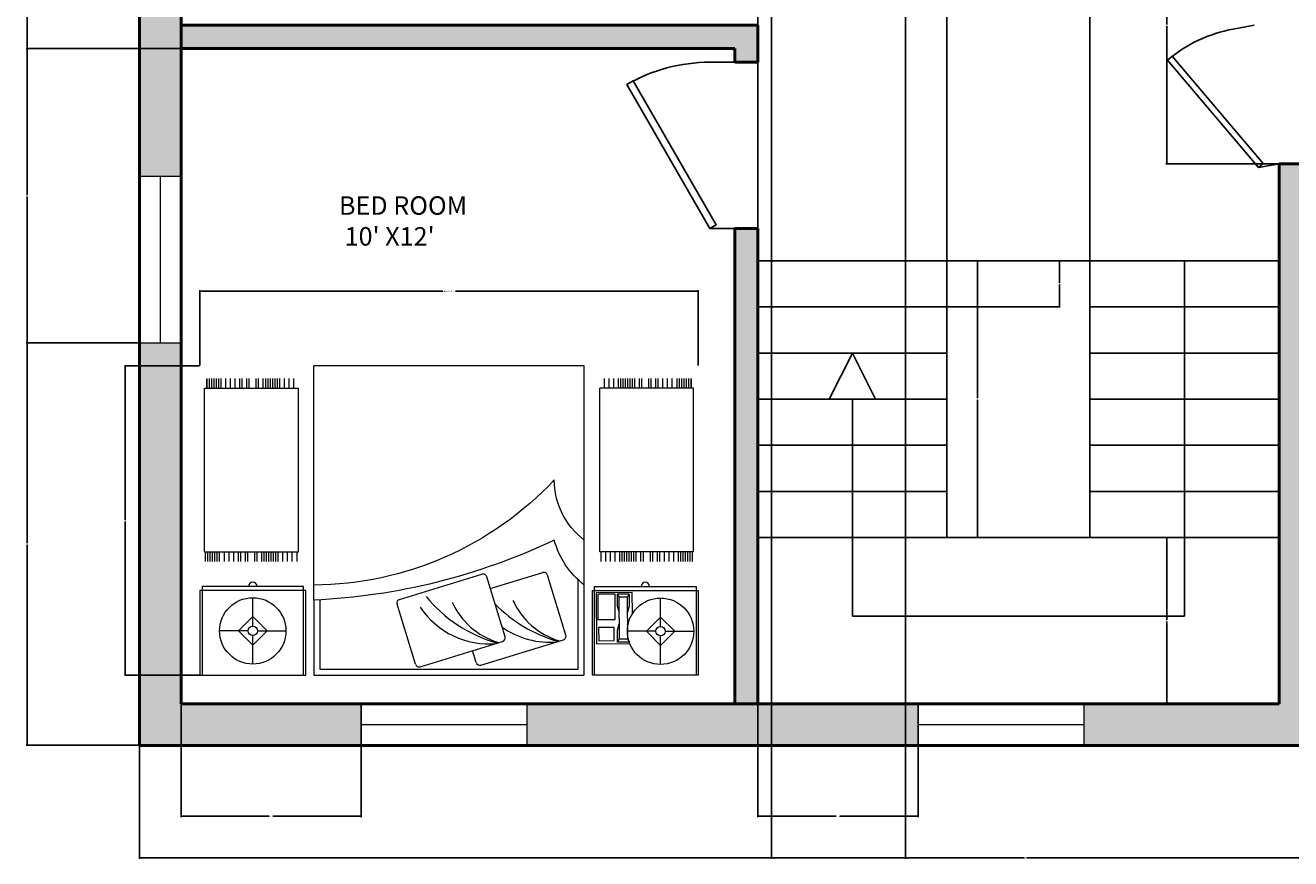
# Model space of a CAD drawing. Units: inches. Extents: x -23 to 411, y -22 to 507.
# Tile 1 of 5: x -23 to 252, y -22 to 159. Entities that reach past the tile are written whole.
import ezdxf

# ---------------------------------------------------------------- set-up
doc = ezdxf.new("R2010")
doc.units = ezdxf.units.IN
doc.header["$MEASUREMENT"] = 0
for name, color, linetype, lineweight in [('A-ANNO-DIMS', 2, 'Continuous', 18), ('A-AREA-IDEN', 7, 'Continuous', 25), ('A-FLOR-STRS', 7, 'Continuous', 25), ('A-WALL', 7, 'Continuous', 50), ('doors', 40, 'Continuous', 25), ('furniture', 220, 'Continuous', 18), ('window', 30, 'Continuous', 18)]:
    doc.layers.add(name, color=color, linetype=linetype, lineweight=lineweight)
doc.layers.add('A-WALL-PATT', color=179, linetype='Continuous', lineweight=13, true_color=0x161b4b)
doc.styles.get("Standard").update_dxf_attribs({"font": 'arial.ttf'})
doc.dimstyles.get("Standard").update_dxf_attribs({"dimtxt": 0.18, "dimasz": 0.18, "dimexe": 0.18, "dimexo": 0.0625, "dimgap": 0.09, "dimtad": 0, "dimtih": 1, "dimtoh": 1, "dimdec": 4, "dimzin": 0, "dimdsep": 46, "dimtxsty": 'Standard', "dimcen": 0.09, "dimadec": 0, "dimazin": 0, "dimtfac": 1, "dimtdec": 4, "dimtofl": 0, "dimtmove": 0, "dimatfit": 3, "dimfxl": 1, "dimtolj": 1, "dimtzin": 0, "dimarcsym": 0})

# ---------------------------------------------------------------- blocks, each defined once
blk = doc.blocks.new('*U6')
for p, q in [((0, 0), (0, -6)), ((40, 0), (40, -6))]:
    blk.add_line(p, q)
blk.add_lwpolyline([(0, 0), (34.64, 20), (35.52, 18.48), (0.87, -1.52)], close=True)
blk.add_arc((0, 0), 40, 0, 30)
blk = doc.blocks.new('3')
for p, q in [((185.8665, 224.6766), (185.8665, 225.2363)), ((185.8665, 225.2363), (186.566, 225.2363)), ((185.8805, 224.6487), (185.8805, 225.2363)), ((186.552, 225.2363), (186.552, 224.6487)), ((186.566, 225.2363), (186.566, 224.6766)), ((186.6199, 225.2363), (186.6199, 224.6399)), ((188.4089, 225.2363), (186.6199, 225.2363)), ((188.4089, 224.7393), (188.4089, 225.2363)), ((188.4627, 225.2363), (188.4627, 224.6766)), ((189.1623, 225.2363), (188.4627, 225.2363)), ((188.4767, 225.2363), (188.4767, 224.6486)), ((189.1483, 224.6486), (189.1483, 225.2363)), ((189.1623, 224.6766), (189.1623, 225.2363)), ((186.1157, 225.1643), (186.1157, 224.9763)), ((187.3034, 225.1683), (186.7581, 225.0015)), ((187.7059, 225.1793), (187.1607, 225.0124)), ((187.3344, 225.1518), (187.3586, 225.073)), ((187.737, 225.1628), (187.8585, 224.7657)), ((188.8125, 225.1618), (188.8125, 224.9738)), ((186.0216, 224.9449), (186.1157, 225.0389)), ((186.1157, 225.0389), (186.2097, 224.9449)), ((186.5397, 225.0274), (186.3193, 225.0266)), ((186.3215, 225.0167), (186.4008, 225.017)), ((186.3334, 224.9969), (186.3215, 225.0167)), ((186.3334, 224.9969), (186.389, 224.9971)), ((186.334, 224.858), (186.3334, 224.9969)), ((186.4008, 225.017), (186.389, 224.9971)), ((186.3895, 224.8582), (186.389, 224.9971)), ((186.4008, 225.017), (186.4011, 224.9376)), ((186.5409, 224.6901), (186.5397, 225.0274)), ((186.7416, 224.9704), (186.8631, 224.5734)), ((187.1442, 224.9814), (187.2657, 224.5843)), ((188.8125, 225.0365), (188.7185, 224.9424)), ((188.9065, 224.9424), (188.8125, 225.0365)), ((186.0843, 224.9449), (185.8963, 224.9449)), ((186.1157, 224.8509), (186.0216, 224.9449)), ((186.2097, 224.9449), (186.1157, 224.8509)), ((186.1157, 224.9136), (186.1157, 224.7256)), ((186.147, 224.9449), (186.335, 224.9449)), ((186.3314, 224.9055), (186.3338, 224.8977)), ((186.4011, 224.9376), (186.3894, 224.8979)), ((188.7812, 224.9424), (188.5931, 224.9424)), ((188.7185, 224.9424), (188.8125, 224.8484)), ((188.8125, 224.8484), (188.9065, 224.9424)), ((188.8125, 224.9111), (188.8125, 224.723)), ((188.8438, 224.9424), (189.0319, 224.9424)), ((186.3023, 224.8297), (186.3029, 224.6892)), ((186.3224, 224.7786), (186.3341, 224.8183)), ((186.334, 224.858), (186.3345, 224.7191)), ((186.3895, 224.8582), (186.39, 224.7193)), ((186.4017, 224.7789), (186.3897, 224.8185)), ((186.3227, 224.6992), (186.3224, 224.7786)), ((186.3345, 224.7191), (186.3227, 224.6992)), ((186.3345, 224.7191), (186.39, 224.7193)), ((186.402, 224.6995), (186.39, 224.7193)), ((186.402, 224.6995), (186.4017, 224.7789)), ((187.842, 224.7347), (187.2967, 224.5678)), ((188.4089, 224.7393), (188.4089, 223.1907)), ((186.566, 224.6766), (185.8665, 224.6766)), ((186.552, 224.6487), (185.8805, 224.6487)), ((186.3029, 224.6892), (186.5409, 224.6901)), ((186.3227, 224.6992), (186.402, 224.6995)), ((186.6199, 224.6399), (186.6199, 223.1907)), ((187.2416, 224.6632), (186.8942, 224.5569)), ((188.4627, 224.6766), (189.1623, 224.6766)), ((188.4767, 224.6486), (189.1483, 224.6486)), ((185.904, 224.4849, -0.9094), (185.904, 224.4204, -0.9094)), ((185.9195, 224.4849, -0.9094), (185.9195, 224.4204, -0.9094)), ((185.9195, 224.4849, -0.9094), (185.9195, 224.4204, -0.9094)), ((185.935, 224.4849, -0.9094), (185.935, 224.4204, -0.9094)), ((185.9505, 224.4849, -0.9094), (185.9505, 224.4204, -0.9094)), ((185.966, 224.4849, -0.9094), (185.966, 224.4204, -0.9094)), ((185.9815, 224.4849, -0.9094), (185.9815, 224.4204, -0.9094)), ((185.997, 224.4849, -0.9094), (185.997, 224.4204, -0.9094)), ((186.028, 224.4849, -0.9094), (186.028, 224.4204, -0.9094)), ((186.059, 224.4849, -0.9094), (186.059, 224.4204, -0.9094)), ((186.09, 224.4849, -0.9094), (186.09, 224.4204, -0.9094)), ((186.09, 224.4849, -0.9094), (186.09, 224.4204, -0.9094)), ((186.121, 224.4849, -0.9094), (186.121, 224.4204, -0.9094)), ((186.1365, 224.4849, -0.9094), (186.1365, 224.4204, -0.9094)), ((186.1675, 224.4849, -0.9094), (186.1675, 224.4204, -0.9094)), ((186.183, 224.4849, -0.9094), (186.183, 224.4204, -0.9094)), ((186.2295, 224.4849, -0.9094), (186.2295, 224.4204, -0.9094)), ((186.245, 224.4849, -0.9094), (186.245, 224.4204, -0.9094)), ((186.276, 224.4849, -0.9094), (186.276, 224.4204, -0.9094)), ((186.2915, 224.4849, -0.9094), (186.2915, 224.4204, -0.9094)), ((186.307, 224.4849, -0.9094), (186.307, 224.4204, -0.9094)), ((186.3225, 224.4849, -0.9094), (186.3225, 224.4204, -0.9094)), ((186.338, 224.4849, -0.9094), (186.338, 224.4204, -0.9094)), ((186.3535, 224.4849, -0.9094), (186.3535, 224.4204, -0.9094)), ((186.369, 224.4849, -0.9094), (186.369, 224.4204, -0.9094)), ((186.3845, 224.4849, -0.9094), (186.3845, 224.4204, -0.9094)), ((186.4155, 224.4849, -0.9094), (186.4155, 224.4204, -0.9094)), ((186.4465, 224.4849, -0.9094), (186.4465, 224.4204, -0.9094)), ((186.4775, 224.4849, -0.9094), (186.4775, 224.4204, -0.9094)), ((186.5085, 224.4849, -0.9094), (186.5085, 224.4204, -0.9094)), ((188.5202, 224.4849, -0.9094), (188.5202, 224.4204, -0.9094)), ((188.5512, 224.4849, -0.9094), (188.5512, 224.4204, -0.9094)), ((188.5822, 224.4849, -0.9094), (188.5822, 224.4204, -0.9094)), ((188.6132, 224.4849, -0.9094), (188.6132, 224.4204, -0.9094)), ((188.6442, 224.4849, -0.9094), (188.6442, 224.4204, -0.9094)), ((188.6597, 224.4849, -0.9094), (188.6597, 224.4204, -0.9094)), ((188.6752, 224.4849, -0.9094), (188.6752, 224.4204, -0.9094)), ((188.6907, 224.4849, -0.9094), (188.6907, 224.4204, -0.9094)), ((188.7062, 224.4849, -0.9094), (188.7062, 224.4204, -0.9094)), ((188.7217, 224.4849, -0.9094), (188.7217, 224.4204, -0.9094)), ((188.7372, 224.4849, -0.9094), (188.7372, 224.4204, -0.9094)), ((188.7527, 224.4849, -0.9094), (188.7527, 224.4204, -0.9094)), ((188.7837, 224.4849, -0.9094), (188.7837, 224.4204, -0.9094)), ((188.7992, 224.4849, -0.9094), (188.7992, 224.4204, -0.9094)), ((188.8457, 224.4849, -0.9094), (188.8457, 224.4204, -0.9094)), ((188.8612, 224.4849, -0.9094), (188.8612, 224.4204, -0.9094)), ((188.8922, 224.4849, -0.9094), (188.8922, 224.4204, -0.9094)), ((188.9077, 224.4849, -0.9094), (188.9077, 224.4204, -0.9094)), ((188.9387, 224.4849, -0.9094), (188.9387, 224.4204, -0.9094)), ((188.9387, 224.4849, -0.9094), (188.9387, 224.4204, -0.9094)), ((188.9697, 224.4849, -0.9094), (188.9697, 224.4204, -0.9094)), ((189.0007, 224.4849, -0.9094), (189.0007, 224.4204, -0.9094)), ((189.0317, 224.4849, -0.9094), (189.0317, 224.4204, -0.9094)), ((189.0472, 224.4849, -0.9094), (189.0472, 224.4204, -0.9094)), ((189.0627, 224.4849, -0.9094), (189.0627, 224.4204, -0.9094)), ((189.0782, 224.4849, -0.9094), (189.0782, 224.4204, -0.9094)), ((189.0937, 224.4849, -0.9094), (189.0937, 224.4204, -0.9094)), ((189.1092, 224.4849, -0.9094), (189.1092, 224.4204, -0.9094)), ((189.1092, 224.4849, -0.9094), (189.1092, 224.4204, -0.9094)), ((189.1247, 224.4849, -0.9094), (189.1247, 224.4204, -0.9094)), ((185.8974, 224.4204, -0.9094), (185.8974, 223.3378, -0.9094)), ((185.8974, 224.4204, -0.9094), (186.5174, 224.4204, -0.9094)), ((186.5174, 224.4204, -0.9094), (186.5174, 223.3378, -0.9094)), ((189.1313, 224.4204, -0.9094), (188.5113, 224.4204, -0.9094)), ((188.5113, 224.4204, -0.9094), (188.5113, 223.3378, -0.9094)), ((189.1313, 224.4204, -0.9094), (189.1313, 223.3378, -0.9094)), ((185.8974, 223.3378, -0.9094), (186.5174, 223.3378, -0.9094)), ((185.9114, 223.3378, -0.9094), (185.9114, 223.2789, -0.9094)), ((185.9114, 223.3378, -0.9094), (185.9114, 223.2789, -0.9094)), ((185.9114, 223.3378, -0.9094), (185.9114, 223.2789, -0.9094)), ((185.9138, 223.3378, -0.9094), (185.9138, 223.2732, -0.9094)), ((185.9293, 223.3378, -0.9094), (185.9293, 223.2732, -0.9094)), ((185.9293, 223.3378, -0.9094), (185.9293, 223.2732, -0.9094)), ((185.9448, 223.3378, -0.9094), (185.9448, 223.2732, -0.9094)), ((185.9603, 223.3378, -0.9094), (185.9603, 223.2732, -0.9094)), ((185.9758, 223.3378, -0.9094), (185.9758, 223.2732, -0.9094)), ((185.9913, 223.3378, -0.9094), (185.9913, 223.2732, -0.9094)), ((186.0068, 223.3378, -0.9094), (186.0068, 223.2732, -0.9094)), ((186.0378, 223.3378, -0.9094), (186.0378, 223.2732, -0.9094)), ((186.0688, 223.3378, -0.9094), (186.0688, 223.2732, -0.9094)), ((186.0998, 223.3378, -0.9094), (186.0998, 223.2732, -0.9094)), ((186.0998, 223.3378, -0.9094), (186.0998, 223.2732, -0.9094)), ((186.1308, 223.3378, -0.9094), (186.1308, 223.2732, -0.9094)), ((186.1463, 223.3378, -0.9094), (186.1463, 223.2732, -0.9094)), ((186.1773, 223.3378, -0.9094), (186.1773, 223.2732, -0.9094)), ((186.1928, 223.3378, -0.9094), (186.1928, 223.2732, -0.9094)), ((186.2393, 223.3378, -0.9094), (186.2393, 223.2732, -0.9094)), ((186.2548, 223.3378, -0.9094), (186.2548, 223.2732, -0.9094)), ((186.2858, 223.3378, -0.9094), (186.2858, 223.2732, -0.9094)), ((186.3013, 223.3378, -0.9094), (186.3013, 223.2732, -0.9094)), ((186.3168, 223.3378, -0.9094), (186.3168, 223.2732, -0.9094)), ((186.3323, 223.3378, -0.9094), (186.3323, 223.2732, -0.9094)), ((186.3478, 223.3378, -0.9094), (186.3478, 223.2732, -0.9094)), ((186.3633, 223.3378, -0.9094), (186.3633, 223.2732, -0.9094)), ((186.3788, 223.3378, -0.9094), (186.3788, 223.2732, -0.9094)), ((186.3943, 223.3378, -0.9094), (186.3943, 223.2732, -0.9094)), ((186.4253, 223.3378, -0.9094), (186.4253, 223.2732, -0.9094)), ((186.4563, 223.3378, -0.9094), (186.4563, 223.2732, -0.9094)), ((186.4873, 223.3378, -0.9094), (186.4873, 223.2732, -0.9094)), ((189.1313, 223.3378, -0.9094), (188.5113, 223.3378, -0.9094)), ((188.5414, 223.3378, -0.9094), (188.5414, 223.2732, -0.9094)), ((188.5724, 223.3378, -0.9094), (188.5724, 223.2732, -0.9094)), ((188.6034, 223.3378, -0.9094), (188.6034, 223.2732, -0.9094)), ((188.6344, 223.3378, -0.9094), (188.6344, 223.2732, -0.9094)), ((188.6499, 223.3378, -0.9094), (188.6499, 223.2732, -0.9094)), ((188.6654, 223.3378, -0.9094), (188.6654, 223.2732, -0.9094)), ((188.6809, 223.3378, -0.9094), (188.6809, 223.2732, -0.9094)), ((188.6964, 223.3378, -0.9094), (188.6964, 223.2732, -0.9094)), ((188.7119, 223.3378, -0.9094), (188.7119, 223.2732, -0.9094)), ((188.7274, 223.3378, -0.9094), (188.7274, 223.2732, -0.9094)), ((188.7429, 223.3378, -0.9094), (188.7429, 223.2732, -0.9094)), ((188.7739, 223.3378, -0.9094), (188.7739, 223.2732, -0.9094)), ((188.7894, 223.3378, -0.9094), (188.7894, 223.2732, -0.9094)), ((188.8359, 223.3378, -0.9094), (188.8359, 223.2732, -0.9094)), ((188.8514, 223.3378, -0.9094), (188.8514, 223.2732, -0.9094)), ((188.8824, 223.3378, -0.9094), (188.8824, 223.2732, -0.9094)), ((188.8979, 223.3378, -0.9094), (188.8979, 223.2732, -0.9094)), ((188.9289, 223.3378, -0.9094), (188.9289, 223.2732, -0.9094)), ((188.9289, 223.3378, -0.9094), (188.9289, 223.2732, -0.9094)), ((188.9599, 223.3378, -0.9094), (188.9599, 223.2732, -0.9094)), ((188.9909, 223.3378, -0.9094), (188.9909, 223.2732, -0.9094)), ((189.022, 223.3378, -0.9094), (189.022, 223.2732, -0.9094)), ((189.0375, 223.3378, -0.9094), (189.0375, 223.2732, -0.9094)), ((189.053, 223.3378, -0.9094), (189.053, 223.2732, -0.9094)), ((189.0685, 223.3378, -0.9094), (189.0685, 223.2732, -0.9094)), ((189.084, 223.3378, -0.9094), (189.084, 223.2732, -0.9094)), ((189.0995, 223.3378, -0.9094), (189.0995, 223.2732, -0.9094)), ((189.0995, 223.3378, -0.9094), (189.0995, 223.2732, -0.9094)), ((189.115, 223.3378, -0.9094), (189.115, 223.2732, -0.9094)), ((189.1173, 223.3378, -0.9094), (189.1173, 223.2789, -0.9094)), ((189.1173, 223.3378, -0.9094), (189.1173, 223.2789, -0.9094)), ((189.1173, 223.3378, -0.9094), (189.1173, 223.2789, -0.9094)), ((186.6199, 223.1907), (188.4089, 223.1907))]:
    blk.add_line(p, q)
blk.add_lwpolyline([(188.3691, 224.7374), (188.3691, 225.1965), (186.6596, 225.1965), (186.6596, 224.606)])
for points in [[(186.4217, 225.0072), (186.422, 224.9199), (186.5252, 224.9202), (186.5249, 225.0075)], [(186.4153, 224.8663), (186.4159, 224.6996), (186.531, 224.7), (186.5304, 224.8667)]]:
    blk.add_lwpolyline(points, close=True)
for points in [[(186.6199, 224.6399, -0.162278), (186.8186, 224.3418, -0.100664), (188.4089, 224.7393, -0.100664)], [(186.6199, 224.3418, -0.236068), (186.8186, 223.9442, -0.205258), (188.4089, 224.6399, -0.205258)]]:
    blk.add_lwpolyline(points, format="xyb")
for centre, radius in [((186.1157, 224.9449), 0.2194), ((188.8125, 224.9424), 0.2194), ((186.1157, 224.9449), 0.0313), ((188.8125, 224.9424), 0.0313)]:
    blk.add_circle(centre, radius)
for centre, radius, start, end in [((187.3107, 225.1446), 0.0248, 17.0142, 107.0142), ((187.7132, 225.1555), 0.0248, 17.0142, 107.0142), ((186.7654, 224.9777), 0.0248, 107.0142, 197.0142), ((186.6474, 224.5408), 0.4873, 24.22087, 73.06906), ((186.8477, 224.4712), 0.5468, 54.68511, 95.16051), ((186.5359, 224.1054), 0.9426, 44.27274, 73.71889), ((187.1679, 224.9887), 0.0248, 107.0142, 197.0142), ((187.0499, 224.5517), 0.4873, 24.22087, 73.06906), ((187.2502, 224.4821), 0.5468, 33.78007, 95.16051), ((186.9385, 224.1164), 0.9426, 39.40233, 73.71889), ((187.8347, 224.7585), 0.0248, 287.0142, 17.0142), ((186.2163, 224.6487), 0.028, 180, 0), ((188.8125, 224.6486), 0.028, 180, 0), ((186.8869, 224.5806), 0.0248, 197.0142, 287.0142), ((187.2894, 224.5916), 0.0248, 197.0142, 287.0142)]:
    blk.add_arc(centre, radius, start, end)
blk = doc.blocks.new('WIN-36IN')
for p, q in [((9, 36), (0, 36)), ((0, 36), (0, 0)), ((4.5, 0), (4.5, 36)), ((9, 0), (9, 36)), ((0, 0), (9, 0)), ((0, 0), (4.5, 0))]:
    blk.add_line(p, q)
blk = doc.blocks.new('*D16')
at = {"layer": 'A-ANNO-DIMS', "color": 0, "lineweight": -2, "transparency": 16777216}
for p, q in [((15.27, 85.16), (15.27, 101.48)), ((123.27, 85.16), (123.27, 101.48)), ((15.45, 101.3), (67.88, 101.3)), ((123.09, 101.3), (70.65, 101.3))]:
    blk.add_line(p, q, dxfattribs=at)
at = {"layer": 'A-ANNO-DIMS', "color": 0, "transparency": 16777216}
for points in [[(15.45, 101.33), (15.45, 101.27), (15.27, 101.3)], [(123.09, 101.33), (123.09, 101.27), (123.27, 101.3)]]:
    blk.add_solid(points, dxfattribs=at)
at = {"layer": 'Defpoints', "color": 0, "transparency": 16777216}
for p in [(15.27, 101.3), (15.27, 85.1), (123.27, 85.1)]:
    blk.add_point(p, dxfattribs=at)
at = {"layer": 'A-ANNO-DIMS', "color": 0, "transparency": 16777216, "insert": (69.27, 101.3), "char_height": 0.18, "attachment_point": 5}
blk.add_mtext('\\A1;BED GROUP 108 TYP.', dxfattribs=at)
blk = doc.blocks.new('*D17')
at = {"layer": 'A-ANNO-DIMS', "color": 0, "lineweight": -2, "transparency": 16777216}
for p, q in [((15.2, 85.1), (-1.11, 85.1)), ((-0.93, 84.92), (-0.93, 51.77)), ((-0.93, 18.25), (-0.93, 51.4)), ((15.2, 18.07), (-1.11, 18.07))]:
    blk.add_line(p, q, dxfattribs=at)
at = {"layer": 'A-ANNO-DIMS', "color": 0, "transparency": 16777216}
for points in [[(-0.96, 84.92), (-0.9, 84.92), (-0.93, 85.1)], [(-0.96, 18.25), (-0.9, 18.25), (-0.93, 18.07)]]:
    blk.add_solid(points, dxfattribs=at)
at = {"layer": 'Defpoints', "color": 0, "transparency": 16777216}
for p in [(15.27, 85.1), (-0.93, 18.07), (15.27, 18.07)]:
    blk.add_point(p, dxfattribs=at)
at = {"layer": 'A-ANNO-DIMS', "color": 0, "transparency": 16777216, "insert": (-0.93, 51.59), "char_height": 0.18, "attachment_point": 5}
blk.add_mtext('\\A1;67 TYP.', dxfattribs=at)
blk = doc.blocks.new('*D28')
at = {"layer": 'A-ANNO-DIMS', "color": 0, "lineweight": -2, "transparency": 16777216}
for p, q in [((2.17, 2.83), (2.17, -21.66)), ((386.17, 2.83), (386.17, -21.66)), ((2.35, -21.48), (193.89, -21.48)), ((385.99, -21.48), (194.46, -21.48))]:
    blk.add_line(p, q, dxfattribs=at)
at = {"layer": 'A-ANNO-DIMS', "color": 0, "transparency": 16777216}
for points in [[(2.35, -21.45), (2.35, -21.51), (2.17, -21.48)], [(385.99, -21.45), (385.99, -21.51), (386.17, -21.48)]]:
    blk.add_solid(points, dxfattribs=at)
at = {"layer": 'Defpoints', "color": 0, "transparency": 16777216}
for p in [(2.17, 2.9), (386.17, 2.9), (386.17, -21.48)]:
    blk.add_point(p, dxfattribs=at)
at = {"layer": 'A-ANNO-DIMS', "color": 0, "transparency": 16777216, "insert": (194.17, -21.48), "char_height": 0.18, "attachment_point": 5}
blk.add_mtext('\\A1;384', dxfattribs=at)
blk = doc.blocks.new('*D38')
at = {"layer": 'A-ANNO-DIMS', "color": 0, "lineweight": -2, "transparency": 16777216}
for p, q in [((2.11, 90.12), (-22.38, 90.12)), ((-22.2, 89.94), (-22.2, 46.69)), ((-22.2, 3.08), (-22.2, 46.33)), ((2.11, 2.9), (-22.38, 2.9))]:
    blk.add_line(p, q, dxfattribs=at)
at = {"layer": 'A-ANNO-DIMS', "color": 0, "transparency": 16777216}
for points in [[(-22.23, 89.94), (-22.17, 89.94), (-22.2, 90.12)], [(-22.23, 3.08), (-22.17, 3.08), (-22.2, 2.9)]]:
    blk.add_solid(points, dxfattribs=at)
at = {"layer": 'Defpoints', "color": 0, "transparency": 16777216}
for p in [(-22.2, 90.12), (2.17, 90.12), (2.17, 2.9)]:
    blk.add_point(p, dxfattribs=at)
at = {"layer": 'A-ANNO-DIMS', "color": 0, "transparency": 16777216, "insert": (-22.2, 46.51), "char_height": 0.18, "attachment_point": 5}
blk.add_mtext('\\A1;87.22', dxfattribs=at)
blk = doc.blocks.new('*D39')
at = {"layer": 'A-ANNO-DIMS', "color": 0, "lineweight": -2, "transparency": 16777216}
for p, q in [((11.11, 153.9), (-22.38, 153.9)), ((-22.2, 153.72), (-22.2, 122.19)), ((-22.2, 90.3), (-22.2, 121.83)), ((2.11, 90.12), (-22.38, 90.12))]:
    blk.add_line(p, q, dxfattribs=at)
at = {"layer": 'A-ANNO-DIMS', "color": 0, "transparency": 16777216}
for points in [[(-22.23, 153.72), (-22.17, 153.72), (-22.2, 153.9)], [(-22.23, 90.3), (-22.17, 90.3), (-22.2, 90.12)]]:
    blk.add_solid(points, dxfattribs=at)
at = {"layer": 'Defpoints', "color": 0, "transparency": 16777216}
for p in [(-22.2, 153.9), (11.17, 153.9), (2.17, 90.12)]:
    blk.add_point(p, dxfattribs=at)
at = {"layer": 'A-ANNO-DIMS', "color": 0, "transparency": 16777216, "insert": (-22.2, 122.01), "char_height": 0.18, "attachment_point": 5}
blk.add_mtext('\\A1;63.78', dxfattribs=at)
blk = doc.blocks.new('*D40')
at = {"layer": 'A-ANNO-DIMS', "color": 0, "lineweight": -2, "transparency": 16777216}
for p, q in [((2.11, 176.25), (-22.38, 176.25)), ((-22.2, 176.07), (-22.2, 165.26)), ((-22.2, 154.08), (-22.2, 164.89)), ((11.11, 153.9), (-22.38, 153.9))]:
    blk.add_line(p, q, dxfattribs=at)
at = {"layer": 'A-ANNO-DIMS', "color": 0, "transparency": 16777216}
for points in [[(-22.23, 176.07), (-22.17, 176.07), (-22.2, 176.25)], [(-22.23, 154.08), (-22.17, 154.08), (-22.2, 153.9)]]:
    blk.add_solid(points, dxfattribs=at)
at = {"layer": 'Defpoints', "color": 0, "transparency": 16777216}
for p in [(-22.2, 176.25), (2.17, 176.25), (11.17, 153.9)]:
    blk.add_point(p, dxfattribs=at)
at = {"layer": 'A-ANNO-DIMS', "color": 0, "transparency": 16777216, "insert": (-22.2, 165.08), "char_height": 0.18, "attachment_point": 5}
blk.add_mtext('\\A1;22.358', dxfattribs=at)
blk = doc.blocks.new('*D45')
at = {"layer": 'A-ANNO-DIMS', "color": 0, "lineweight": -2, "transparency": 16777216}
for p, q in [((136.17, 107.96), (136.17, 507.45)), ((177.17, 107.96), (177.17, 507.45)), ((136.35, 507.27), (156.47, 507.27)), ((176.99, 507.27), (156.88, 507.27))]:
    blk.add_line(p, q, dxfattribs=at)
at = {"layer": 'A-ANNO-DIMS', "color": 0, "transparency": 16777216}
for points in [[(136.35, 507.3), (136.35, 507.24), (136.17, 507.27)], [(176.99, 507.3), (176.99, 507.24), (177.17, 507.27)]]:
    blk.add_solid(points, dxfattribs=at)
at = {"layer": 'Defpoints', "color": 0, "transparency": 16777216}
for p in [(177.17, 507.27), (136.17, 107.9), (177.17, 107.9)]:
    blk.add_point(p, dxfattribs=at)
at = {"layer": 'A-ANNO-DIMS', "color": 0, "transparency": 16777216, "insert": (156.67, 507.27), "char_height": 0.18, "attachment_point": 5}
blk.add_mtext('\\A1;41', dxfattribs=at)
blk = doc.blocks.new('*D46')
at = {"layer": 'A-ANNO-DIMS', "color": 0, "lineweight": -2, "transparency": 16777216}
for p, q in [((177.17, 107.96), (177.17, 507.45)), ((208.17, 107.96), (208.17, 507.45)), ((177.35, 507.27), (192.47, 507.27)), ((207.99, 507.27), (192.88, 507.27))]:
    blk.add_line(p, q, dxfattribs=at)
at = {"layer": 'A-ANNO-DIMS', "color": 0, "transparency": 16777216}
for points in [[(177.35, 507.3), (177.35, 507.24), (177.17, 507.27)], [(207.99, 507.3), (207.99, 507.24), (208.17, 507.27)]]:
    blk.add_solid(points, dxfattribs=at)
at = {"layer": 'Defpoints', "color": 0, "transparency": 16777216}
for p in [(208.17, 507.27), (177.17, 107.9), (208.17, 107.9)]:
    blk.add_point(p, dxfattribs=at)
at = {"layer": 'A-ANNO-DIMS', "color": 0, "transparency": 16777216, "insert": (192.67, 507.27), "char_height": 0.18, "attachment_point": 5}
blk.add_mtext('\\A1;31', dxfattribs=at)
blk = doc.blocks.new('*D47')
at = {"layer": 'A-ANNO-DIMS', "color": 0, "lineweight": -2, "transparency": 16777216}
for p, q in [((208.11, 107.9), (183.62, 107.9)), ((183.8, 107.72), (183.8, 78.08)), ((183.8, 48.08), (183.8, 77.72)), ((208.11, 47.9), (183.62, 47.9))]:
    blk.add_line(p, q, dxfattribs=at)
at = {"layer": 'A-ANNO-DIMS', "color": 0, "transparency": 16777216}
for points in [[(183.77, 107.72), (183.83, 107.72), (183.8, 107.9)], [(183.77, 48.08), (183.83, 48.08), (183.8, 47.9)]]:
    blk.add_solid(points, dxfattribs=at)
at = {"layer": 'Defpoints', "color": 0, "transparency": 16777216}
for p in [(183.8, 107.9), (208.17, 107.9), (208.17, 47.9)]:
    blk.add_point(p, dxfattribs=at)
at = {"layer": 'A-ANNO-DIMS', "color": 0, "transparency": 16777216, "insert": (183.8, 77.9), "char_height": 0.18, "attachment_point": 5}
blk.add_mtext('\\A1;60', dxfattribs=at)
blk = doc.blocks.new('*D48')
at = {"layer": 'A-ANNO-DIMS', "color": 0, "lineweight": -2, "transparency": 16777216}
for p, q in [((177.24, 107.9), (201.73, 107.9)), ((201.55, 107.72), (201.55, 103.08)), ((201.55, 98.08), (201.55, 102.72)), ((177.24, 97.9), (201.73, 97.9))]:
    blk.add_line(p, q, dxfattribs=at)
at = {"layer": 'A-ANNO-DIMS', "color": 0, "transparency": 16777216}
for points in [[(201.52, 107.72), (201.58, 107.72), (201.55, 107.9)], [(201.52, 98.08), (201.58, 98.08), (201.55, 97.9)]]:
    blk.add_solid(points, dxfattribs=at)
at = {"layer": 'Defpoints', "color": 0, "transparency": 16777216}
for p in [(177.17, 107.9), (177.17, 97.9), (201.55, 97.9)]:
    blk.add_point(p, dxfattribs=at)
at = {"layer": 'A-ANNO-DIMS', "color": 0, "transparency": 16777216, "insert": (201.55, 102.9), "char_height": 0.18, "attachment_point": 5}
blk.add_mtext('\\A1;10', dxfattribs=at)
blk = doc.blocks.new('*D49')
at = {"layer": 'A-ANNO-DIMS', "color": 0, "lineweight": -2, "transparency": 16777216}
for p, q in [((249.11, 47.9), (224.62, 47.9)), ((224.8, 47.72), (224.8, 30.08)), ((224.8, 12.08), (224.8, 29.72)), ((249.11, 11.9), (224.62, 11.9))]:
    blk.add_line(p, q, dxfattribs=at)
at = {"layer": 'A-ANNO-DIMS', "color": 0, "transparency": 16777216}
for points in [[(224.77, 47.72), (224.83, 47.72), (224.8, 47.9)], [(224.77, 12.08), (224.83, 12.08), (224.8, 11.9)]]:
    blk.add_solid(points, dxfattribs=at)
at = {"layer": 'Defpoints', "color": 0, "transparency": 16777216}
for p in [(224.8, 47.9), (249.17, 47.9), (249.17, 11.9)]:
    blk.add_point(p, dxfattribs=at)
at = {"layer": 'A-ANNO-DIMS', "color": 0, "transparency": 16777216, "insert": (224.8, 29.9), "char_height": 0.18, "attachment_point": 5}
blk.add_mtext('\\A1;36', dxfattribs=at)
blk = doc.blocks.new('*D50')
at = {"layer": 'A-ANNO-DIMS', "color": 0, "lineweight": -2, "transparency": 16777216}
for p, q in [((139.17, 372.83), (139.17, -21.66)), ((168.17, 372.83), (168.17, -21.66)), ((139.35, -21.48), (153.45, -21.48)), ((167.99, -21.48), (153.9, -21.48))]:
    blk.add_line(p, q, dxfattribs=at)
at = {"layer": 'A-ANNO-DIMS', "color": 0, "transparency": 16777216}
for points in [[(139.35, -21.45), (139.35, -21.51), (139.17, -21.48)], [(167.99, -21.45), (167.99, -21.51), (168.17, -21.48)]]:
    blk.add_solid(points, dxfattribs=at)
at = {"layer": 'Defpoints', "color": 0, "transparency": 16777216}
for p in [(139.17, 372.9), (168.17, 372.9), (168.17, -21.48)]:
    blk.add_point(p, dxfattribs=at)
at = {"layer": 'A-ANNO-DIMS', "color": 0, "transparency": 16777216, "insert": (153.67, -21.48), "char_height": 0.18, "attachment_point": 5}
blk.add_mtext('\\A1;29', dxfattribs=at)
blk = doc.blocks.new('*D52')
at = {"layer": 'A-ANNO-DIMS', "color": 0, "lineweight": -2, "transparency": 16777216}
for p, q in [((249.11, 188.9), (224.62, 188.9)), ((224.8, 188.72), (224.8, 159.08)), ((224.8, 129.08), (224.8, 158.72)), ((249.11, 128.9), (224.62, 128.9))]:
    blk.add_line(p, q, dxfattribs=at)
at = {"layer": 'A-ANNO-DIMS', "color": 0, "transparency": 16777216}
for points in [[(224.77, 188.72), (224.83, 188.72), (224.8, 188.9)], [(224.77, 129.08), (224.83, 129.08), (224.8, 128.9)]]:
    blk.add_solid(points, dxfattribs=at)
at = {"layer": 'Defpoints', "color": 0, "transparency": 16777216}
for p in [(224.8, 188.9), (249.17, 188.9), (249.17, 128.9)]:
    blk.add_point(p, dxfattribs=at)
at = {"layer": 'A-ANNO-DIMS', "color": 0, "transparency": 16777216, "insert": (224.8, 158.9), "char_height": 0.18, "attachment_point": 5}
blk.add_mtext('\\A1;60', dxfattribs=at)
blk = doc.blocks.new('*D58')
at = {"layer": 'A-ANNO-DIMS', "color": 0, "lineweight": -2, "transparency": 16777216}
for p, q in [((11.17, 11.83), (11.17, -12.66)), ((50.21, 11.83), (50.21, -12.66)), ((11.35, -12.48), (30.3, -12.48)), ((50.03, -12.48), (31.09, -12.48))]:
    blk.add_line(p, q, dxfattribs=at)
at = {"layer": 'A-ANNO-DIMS', "color": 0, "transparency": 16777216}
for points in [[(11.35, -12.45), (11.35, -12.51), (11.17, -12.48)], [(50.03, -12.45), (50.03, -12.51), (50.21, -12.48)]]:
    blk.add_solid(points, dxfattribs=at)
at = {"layer": 'Defpoints', "color": 0, "transparency": 16777216}
for p in [(11.17, 11.9), (50.21, 11.9), (11.17, -12.48)]:
    blk.add_point(p, dxfattribs=at)
at = {"layer": 'A-ANNO-DIMS', "color": 0, "transparency": 16777216, "insert": (30.69, -12.48), "char_height": 0.18, "attachment_point": 5}
blk.add_mtext('\\A1;39.04', dxfattribs=at)
blk = doc.blocks.new('*D59')
at = {"layer": 'A-ANNO-DIMS', "color": 0, "lineweight": -2, "transparency": 16777216}
for p, q in [((136.17, 11.83), (136.17, -12.66)), ((170.92, 11.83), (170.92, -12.66)), ((136.35, -12.48), (153.15, -12.48)), ((170.74, -12.48), (153.94, -12.48))]:
    blk.add_line(p, q, dxfattribs=at)
at = {"layer": 'A-ANNO-DIMS', "color": 0, "transparency": 16777216}
for points in [[(136.35, -12.45), (136.35, -12.51), (136.17, -12.48)], [(170.74, -12.45), (170.74, -12.51), (170.92, -12.48)]]:
    blk.add_solid(points, dxfattribs=at)
at = {"layer": 'Defpoints', "color": 0, "transparency": 16777216}
for p in [(136.17, 11.9), (170.92, 11.9), (136.17, -12.48)]:
    blk.add_point(p, dxfattribs=at)
at = {"layer": 'A-ANNO-DIMS', "color": 0, "transparency": 16777216, "insert": (153.55, -12.48), "char_height": 0.18, "attachment_point": 5}
blk.add_mtext('\\A1;34.74', dxfattribs=at)

msp = doc.modelspace()

# ---------------------------------------------------------------- hatches: boundary and pattern name
at = {"layer": 'A-WALL-PATT'}
h = msp.add_hatch(color=256, dxfattribs=at)
h.dxf.hatch_style = 1
h.paths.add_polyline_path([(37.3453, 482.8972), (2.1746, 482.8972), (2.1746, 414.9823), (11.1746, 414.9823), (11.1746, 473.8972), (37.3453, 473.8972)])
h.paths.add_polyline_path([(149.2817, 482.8972), (73.3453, 482.8972), (73.3453, 473.8972), (131.1746, 473.8972), (131.1746, 356.8972), (136.1746, 356.8972), (136.1746, 372.8972), (139.1746, 372.8972), (139.1746, 377.8972), (136.1746, 377.8972), (136.1746, 473.8972), (149.2817, 473.8972)])
h.paths.add_polyline_path([(209.1361, 482.8972), (173.2817, 482.8972), (173.2817, 473.8972), (190.1746, 473.8972), (190.1746, 377.8972), (168.1746, 377.8972), (168.1746, 372.8972), (249.1746, 372.8972), (249.1746, 356.8972), (254.1746, 356.8972), (254.1746, 380.8972), (249.1746, 380.8972), (249.1746, 377.8972), (195.1746, 377.8972), (195.1746, 473.8972), (209.1361, 473.8972)])
h.paths.add_polyline_path([(309.9724, 482.8972), (233.1361, 482.8972), (233.1361, 473.8972), (249.1746, 473.8972), (249.1746, 409.8972), (254.1746, 409.8972), (254.1746, 473.8972), (309.9724, 473.8972)])
h.paths.add_polyline_path([(386.1746, 482.8972), (345.9724, 482.8972), (345.9724, 473.8972), (377.1746, 473.8972), (377.1746, 445.6454), (386.1746, 445.6454)])
h.paths.add_polyline_path([(386.1746, 409.6454), (377.1746, 409.6454), (377.1746, 317.8972), (254.1746, 317.8972), (254.1746, 320.8972), (249.1746, 320.8972), (249.1746, 317.8972), (249.1746, 235.8972), (254.1746, 235.8972), (254.1746, 312.8972), (377.1746, 312.8972), (377.1746, 281.3732), (386.1746, 281.3732)])
h.paths.add_polyline_path([(386.1746, 245.3732), (377.1746, 245.3732), (377.1746, 196.8972), (254.1746, 196.8972), (254.1746, 199.8972), (249.1746, 199.8972), (249.1746, 196.8972), (249.1746, 188.8972), (254.1746, 188.8972), (254.1746, 191.8972), (264.1746, 191.8972), (377.1746, 191.8972), (377.1746, 11.8972), (377.1746, 2.8972), (386.1746, 2.8972)])
h.paths.add_polyline_path([(254.1746, 128.8972), (249.1746, 128.8972), (249.1746, 11.8972), (206.9157, 11.8972), (206.9157, 2.8972), (254.1746, 2.8972)])
h.paths.add_polyline_path([(170.9157, 11.8972), (86.2116, 11.8972), (86.2116, 2.8972), (170.9157, 2.8972)])
h.paths.add_polyline_path([(136.1746, 114.8972), (131.1746, 114.8972), (131.1746, 11.8972), (136.1746, 11.8972)])
h.paths.add_polyline_path([(50.2116, 11.8972), (11.1746, 11.8972), (11.1746, 90.1201), (2.1746, 90.1201), (2.1746, 2.8972), (50.2116, 2.8972)])
h.paths.add_polyline_path([(11.1746, 176.2548), (2.1746, 176.2548), (2.1746, 126.1201), (11.1746, 126.1201)])
h.paths.add_polyline_path([(136.1746, 158.8972), (11.1746, 158.8972), (11.1746, 153.8972), (131.1746, 153.8972), (131.1746, 150.8972), (136.1746, 150.8972)])
h.paths.add_polyline_path([(11.1746, 269.5052), (2.1746, 269.5052), (2.1746, 212.2548), (11.1746, 212.2548)])
h.paths.add_polyline_path([(11.1746, 378.9823), (2.1746, 378.9823), (2.1746, 305.5052), (11.1746, 305.5052), (11.1746, 312.8972), (136.1746, 312.8972), (136.1746, 320.8972), (131.1746, 320.8972), (131.1746, 317.8972), (11.1746, 317.8972)])

# ---------------------------------------------------------------- linework, layer by layer
at = {"layer": 'A-FLOR-STRS'}
for p, q in [((136.1746, 107.8972), (177.1746, 107.8972)), ((136.1746, 107.8972), (177.1746, 107.8972)), ((177.1746, 107.8972), (177.1746, 47.8972)), ((208.1746, 107.8972), (249.1746, 107.8972)), ((249.1746, 107.8972), (208.1746, 107.8972)), ((208.1746, 107.8972), (208.1746, 47.8972)), ((228.6746, 107.8972), (228.6746, 35.3776)), ((136.1746, 97.8972), (177.1746, 97.8972)), ((208.1746, 97.8972), (249.1746, 97.8972)), ((136.1746, 87.8972), (177.1746, 87.8972)), ((151.6746, 77.8972), (156.6746, 87.8972)), ((161.6746, 77.8972), (156.6746, 87.8972)), ((208.1746, 87.8972), (249.1746, 87.8972)), ((136.1746, 77.8972), (177.1746, 77.8972)), ((136.1746, 77.8972), (177.1746, 77.8972)), ((156.6746, 77.8972), (151.6746, 77.8972)), ((156.6746, 77.8972), (156.6746, 47.8972)), ((156.6746, 77.8972), (161.6746, 77.8972)), ((208.1746, 77.8972), (249.1746, 77.8972)), ((208.1746, 77.8972), (249.1746, 77.8972)), ((136.1746, 67.8972), (177.1746, 67.8972)), ((208.1746, 67.8972), (249.1746, 67.8972)), ((136.1746, 57.8972), (177.1746, 57.8972)), ((208.1746, 57.8972), (249.1746, 57.8972)), ((136.1746, 11.8972), (136.1746, 47.8972)), ((136.1746, 47.8972), (249.1746, 47.8972)), ((156.6746, 47.8972), (156.6746, 30.8972)), ((228.6746, 30.8972), (228.6746, 35.3776)), ((156.6746, 30.8972), (228.6746, 30.8972))]:
    msp.add_line(p, q, dxfattribs=at)
at = {"layer": 'A-WALL'}
for p, q in [((11.1746, 11.8972), (11.1746, 191.8972)), ((11.1746, 158.8972), (136.1746, 158.8972)), ((136.1746, 150.8972), (136.1746, 158.8972)), ((11.1746, 153.8972), (131.1746, 153.8972)), ((131.1746, 150.8972), (131.1746, 153.8972)), ((131.1746, 153.8972), (131.1746, 150.8972)), ((131.1746, 150.8972), (136.1746, 150.8972)), ((249.1746, 11.8972), (249.1746, 128.8972)), ((249.1746, 128.8972), (254.1746, 128.8972)), ((131.1746, 11.8972), (131.1746, 114.8972)), ((136.1746, 114.8972), (131.1746, 114.8972)), ((136.1746, 11.8972), (136.1746, 114.8972)), ((249.1746, 11.8972), (11.1746, 11.8972))]:
    msp.add_line(p, q, dxfattribs=at)
msp.add_lwpolyline([(254.1746, 2.8972), (2.1746, 2.8972), (2.1746, 482.8972), (386.1746, 482.8972), (386.1746, 2.8972), (377.1746, 2.8972)], dxfattribs=at)

# ---------------------------------------------------------------- block references
at = {"layer": 'doors'}
for p, xscale, yscale, zscale, rotation in [((244.6746, 128.0817), 0.7622159057711964, 0.7622159057711964, 0.7622159057711964, 100.2717207928814), ((125.7746, 114.8972), 0.9, 0.9, 0.9, 90)]:
    msp.add_blockref('*U6', p, dxfattribs=dict(at, xscale=xscale, yscale=yscale, zscale=zscale, rotation=rotation))
at = {"layer": 'furniture', "xscale": 32.76894482774335, "yscale": 32.76894482774335, "zscale": 32.76894482774335, "rotation": 180}
msp.add_blockref('3', (6213.9154, 7398.8253), dxfattribs=at)
at = {"layer": 'window'}
for p, rotation in [((11.1741, 126.1203), 180), ((50.2114, 11.8967), 270), ((170.9155, 11.8967), 270)]:
    msp.add_blockref('WIN-36IN', p, dxfattribs=dict(at, rotation=rotation))

# ---------------------------------------------------------------- texts
at = {"layer": 'A-AREA-IDEN', "insert": (45.4014, 121.8448), "char_height": 4, "attachment_point": 1}
msp.add_mtext_dynamic_manual_height_columns("BED ROOM\\P 10' X12'", width=61.991846, gutter_width=1, heights=[0], dxfattribs=at)

# ---------------------------------------------------------------- dimensions: what is measured, and where the dimension line sits
at = {"layer": 'A-ANNO-DIMS'}
for base, p1, p2, picture, middle in [((177.1746, 507.2747), (136.1746, 107.8972), (177.1746, 107.8972), '*D45', (156.6746, 507.2747)), ((208.1746, 507.2747), (177.1746, 107.8972), (208.1746, 107.8972), '*D46', (192.6746, 507.2747)), ((168.1746, -21.4803), (139.1746, 372.8972), (168.1746, 372.8972), '*D50', (153.6746, -21.4803)), ((386.1746, -21.4803), (2.1746, 2.8972), (386.1746, 2.8972), '*D28', (194.1746, -21.4803))]:
    dim = msp.add_linear_dim(base=base, p1=p1, p2=p2, dimstyle='Standard', override={"dimdec": 0, "dimlfac": 1, "dimrnd": 0, "dimzin": 0, "dimdsep": 46, "dimlunit": 2}, dxfattribs=at)
    dim.commit()
    dim.dimension.update_dxf_attribs({"geometry": picture, "text_midpoint": middle})
for base, p1, p2, angle, override, picture, middle in [((224.7971, 188.8972), (249.1746, 128.8972), (249.1746, 188.8972), 90, {"dimdec": 0, "dimlfac": 1, "dimrnd": 0, "dimzin": 0, "dimdsep": 46, "dimlunit": 2}, '*D52', (224.7971, 158.8972)), ((-22.2029, 176.2548), (11.1746, 153.8972), (2.1746, 176.2548), 90, {"dimdec": 3, "dimlfac": 1, "dimrnd": 0, "dimzin": 0, "dimdsep": 46, "dimlunit": 2}, '*D40', (-22.2029, 165.076)), ((-22.2029, 153.8972), (2.1746, 90.1201), (11.1746, 153.8972), 90, {"dimdec": 2, "dimlfac": 1, "dimrnd": 0, "dimzin": 0, "dimdsep": 46, "dimlunit": 2}, '*D39', (-22.2029, 122.0086)), ((201.5521, 97.8972), (177.1746, 107.8972), (177.1746, 97.8972), 270, {"dimdec": 0, "dimlfac": 1, "dimrnd": 0, "dimzin": 0, "dimdsep": 46, "dimlunit": 2}, '*D48', (201.5521, 102.8972)), ((183.7971, 107.8972), (208.1746, 47.8972), (208.1746, 107.8972), 90, {"dimdec": 0, "dimlfac": 1, "dimrnd": 0, "dimzin": 0, "dimdsep": 46, "dimlunit": 2}, '*D47', (183.7971, 77.8972)), ((-22.2029, 90.1201), (2.1746, 2.8972), (2.1746, 90.1201), 90, {"dimdec": 2, "dimlfac": 1, "dimrnd": 0, "dimzin": 0, "dimdsep": 46, "dimlunit": 2}, '*D38', (-22.2029, 46.5086)), ((224.7971, 47.8972), (249.1746, 11.8972), (249.1746, 47.8972), 90, {"dimdec": 0, "dimlfac": 1, "dimrnd": 0, "dimzin": 0, "dimdsep": 46, "dimlunit": 2}, '*D49', (224.7971, 29.8972)), ((11.1746, -12.4803), (50.2116, 11.8972), (11.1746, 11.8972), 180, {"dimdec": 2, "dimlfac": 1, "dimrnd": 0, "dimzin": 0, "dimdsep": 46, "dimlunit": 2}, '*D58', (30.6931, -12.4803)), ((136.1746, -12.4803), (170.9157, 11.8972), (136.1746, 11.8972), 180, {"dimdec": 2, "dimlfac": 1, "dimrnd": 0, "dimzin": 0, "dimdsep": 46, "dimlunit": 2}, '*D59', (153.5451, -12.4803))]:
    dim = msp.add_linear_dim(base=base, p1=p1, p2=p2, angle=angle, dimstyle='Standard', override=override, dxfattribs=at)
    dim.commit()
    dim.dimension.update_dxf_attribs({"geometry": picture, "text_midpoint": middle})
for base, p1, p2, angle, text, picture, middle in [((15.2664, 101.3024), (123.2664, 85.1024), (15.2664, 85.1024), 180, 'BED GROUP <> TYP.', '*D16', (69.2664, 101.3024)), ((-0.9336, 18.0705), (15.2664, 85.1024), (15.2664, 18.0705), 270, '<> TYP.', '*D17', (-0.9336, 51.5864))]:
    dim = msp.add_linear_dim(base=base, p1=p1, p2=p2, angle=angle, text=text, dimstyle='Standard', override={"dimdec": 0, "dimlfac": 1, "dimrnd": 0, "dimzin": 0, "dimdsep": 46, "dimlunit": 2}, dxfattribs=at)
    dim.commit()
    dim.dimension.update_dxf_attribs({"geometry": picture, "text_midpoint": middle})

doc.saveas('drawing.dxf')
